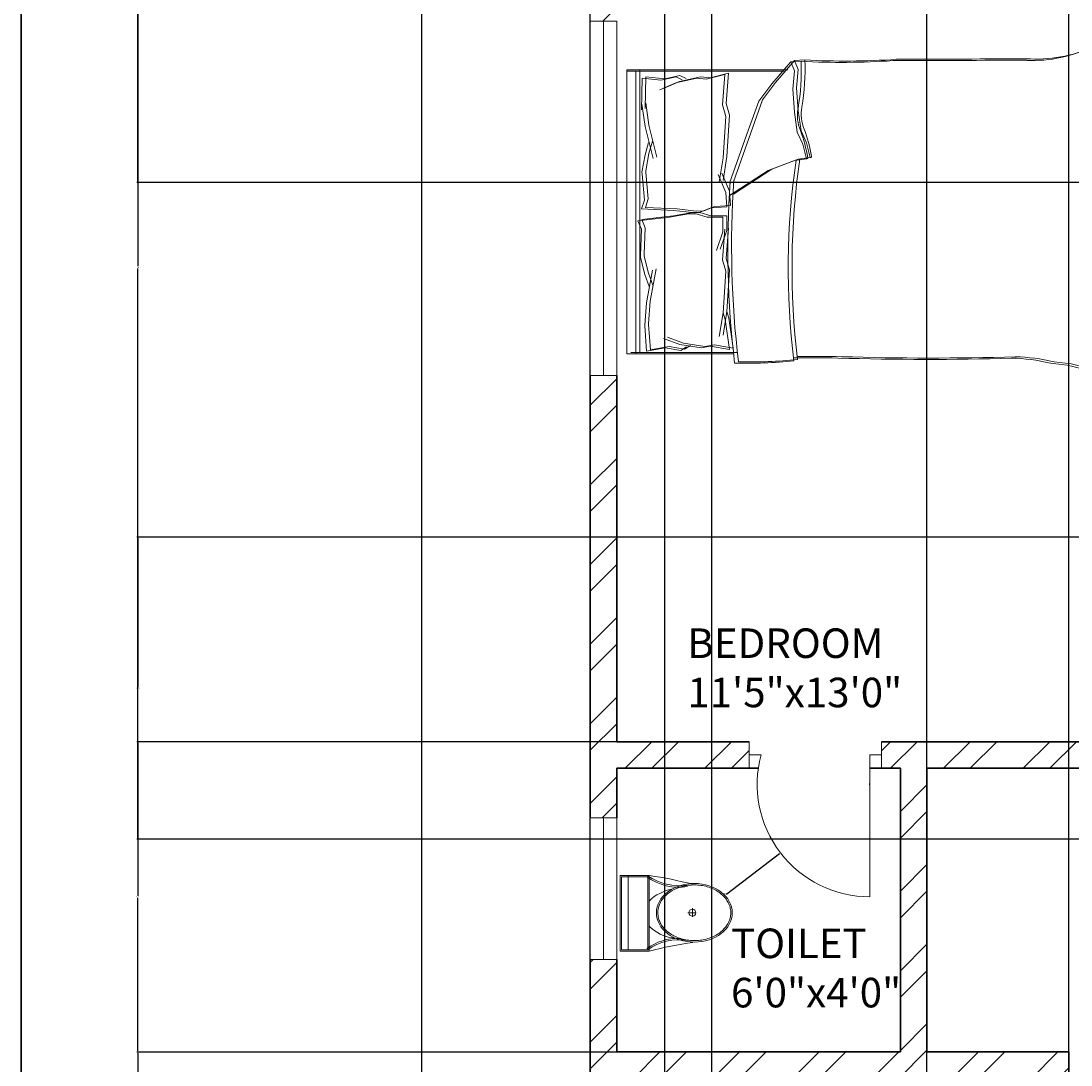
# Model space of a CAD drawing. Units: inches. Extents: x 2008 to 2657, y 1077 to 2165.
# Tile 10 of 16: x 2008 to 2186, y 1845 to 2022. Entities that reach past the tile are written whole.
import ezdxf

# ---------------------------------------------------------------- set-up
doc = ezdxf.new("R2010")
doc.units = ezdxf.units.IN
for name, color, linetype, lineweight in [('A-ANNO-DIMS', 2, 'Continuous', 18), ('A-ANNO-TTLB', 7, 'Continuous', 35), ('A-AREA-IDEN', 4, 'Continuous', 18), ('A-DOOR', 11, 'Continuous', 18), ('A-FLOR-FIXT', 8, 'Continuous', 18), ('A-FURN', 8, 'Continuous', 13), ('A-GLAZ', 191, 'Continuous', 18), ('A-WALL', 7, 'Continuous', 35)]:
    doc.layers.add(name, color=color, linetype=linetype, lineweight=lineweight)
doc.layers.add('A-WALL-PATT', color=30, linetype='Continuous', lineweight=13, true_color=0xf8991e)
doc.styles.get("Standard").update_dxf_attribs({"font": 'arial.ttf'})
doc.dimstyles.get("Standard").update_dxf_attribs({"dimtxt": 0.18, "dimasz": 0.18, "dimexe": 0.18, "dimexo": 0.0625, "dimgap": 0.09, "dimtad": 0, "dimtih": 1, "dimtoh": 1, "dimdec": 4, "dimzin": 0, "dimdsep": 46, "dimtxsty": 'Standard', "dimcen": 0.09, "dimadec": 0, "dimazin": 0, "dimtfac": 1, "dimtdec": 4, "dimtofl": 0, "dimtmove": 0, "dimatfit": 3, "dimfxl": 1, "dimtolj": 1, "dimtzin": 0, "dimarcsym": 0})

# ---------------------------------------------------------------- blocks, each defined once
blk = doc.blocks.new('A$C31115884')
for p, q in [((257.5, 466.4), (257.5, 523.2)), ((283.1, 497.7), (223.4, 497.7)), ((0, 200), (0, 0)), ((520, 200), (0, 200)), ((10, 190), (10, 10)), ((510, 190), (10, 190)), ((510, 10), (510, 190)), ((520, 0), (520, 200)), ((510, 54.5), (0, 54.5)), ((10, 10), (510, 10)), ((0, 0), (520, 0))]:
    blk.add_line(p, q)
blk.add_circle((255.6, 496.4), 23.6)
for centre, radius, start, end in [((2777.7, -204.6), 2807, 165.4549, 171.71327), ((-294.5, 403.3), 364.7, 324.20913, 9.34987), ((-294.5, 403.3), 374.7, 324.20913, 9.34987), ((805.8, 403.3), 364.7, 170.65013, 215.79087), ((3237, 905), 2807, 188.28673, 194.5451), ((139.5, 406.2), 293.5, 315.84364, 2.65635), ((805.8, 403.3), 374.7, 179.20365, 215.79087), ((383.6, 406.2), 293.5, 190.27735, 224.15636)]:
    blk.add_arc(centre, radius, start, end)
blk.add_ellipse((256.2, 509.9), major_axis=(0, -260.7), ratio=0.772727)
blk.add_open_spline([(256.2, 259.2), (263.1, 259.2), (270, 259.7), (287.8, 262.3), (298.7, 265.1), (319.9, 273.1), (330.2, 278.4), (350.1, 291.1), (359.7, 298.7), (377.7, 315.9), (386.2, 325.5), (401.7, 346.6), (408.8, 358.1), (421.3, 382.5), (426.8, 395.5), (435.9, 422.4), (439.5, 436.4), (444.8, 465.1), (446.5, 479.7), (447.9, 509.2), (447.6, 524), (445, 553.3), (442.7, 567.8), (436.3, 596), (432.1, 609.7), (421.9, 636), (416, 648.6), (402.5, 672.1), (395, 683), (378.6, 703), (369.8, 712.1), (351.1, 728), (341.3, 734.8), (320.9, 746.2), (310.4, 750.7), (288.9, 757.3), (278, 759.4), (256, 761), (245, 760.6), (223.1, 757.2), (212.3, 754.3), (191.1, 746.1), (180.8, 740.7), (160.9, 727.8), (151.4, 720.1), (133.5, 702.7), (125.1, 693), (109.6, 671.7), (102.6, 660.2), (90.2, 635.7), (84.9, 622.7), (76, 595.6), (72.4, 581.6), (67.2, 552.9), (65.6, 538.2), (64.4, 508.8), (64.8, 494), (67.5, 464.7), (69.9, 450.2), (76.6, 422), (80.8, 408.3), (91.1, 382.2), (97.2, 369.7), (110.8, 346.3), (118.4, 335.4), (134.8, 315.6), (143.7, 306.7), (162.4, 290.9), (172.3, 284.2), (192.8, 273), (203.3, 268.6), (224.8, 262.2), (235.8, 260.2), (249.9, 259.3), (253, 259.2), (256.2, 259.2)], degree=3, knots=[0, 0, 0, 0, 0.110105, 0.110105, 0.285049, 0.285049, 0.459994, 0.459994, 0.634938, 0.634938, 0.809882, 0.809882, 0.984827, 0.984827, 1.159771, 1.159771, 1.334715, 1.334715, 1.50966, 1.50966, 1.684604, 1.684604, 1.859549, 1.859549, 2.034493, 2.034493, 2.209437, 2.209437, 2.384382, 2.384382, 2.559326, 2.559326, 2.73427, 2.73427, 2.909215, 2.909215, 3.084159, 3.084159, 3.259103, 3.259103, 3.434048, 3.434048, 3.608992, 3.608992, 3.783936, 3.783936, 3.958881, 3.958881, 4.133825, 4.133825, 4.30877, 4.30877, 4.483714, 4.483714, 4.658658, 4.658658, 4.833603, 4.833603, 5.008547, 5.008547, 5.183491, 5.183491, 5.358436, 5.358436, 5.53338, 5.53338, 5.708324, 5.708324, 5.883269, 5.883269, 6.058213, 6.058213, 6.233158, 6.233158, 6.283185, 6.283185, 6.283185, 6.283185])
blk = doc.blocks.new('BED-DOUBLE')
for p, q in [((27.75, 52.87), (24.5, 49.16)), ((27.75, 52.87), (24.5, 49.16)), ((28.39, 53.1), (25.14, 49.39)), ((28.39, 53.1), (25.14, 49.39)), ((29.49, 52.95), (27.75, 52.87, 3.87)), ((29.49, 52.95), (27.75, 52.87, 3.87)), ((28.37, 51.33), (27.75, 52.87)), ((28.37, 51.33), (27.75, 52.87)), ((30.13, 53.18), (28.39, 53.1, 3.87)), ((30.13, 53.18), (28.39, 53.1, 3.87)), ((29, 51.56), (28.39, 53.1)), ((29, 51.56), (28.39, 53.1)), ((28.7, 48.46), (29, 51.56)), ((28.7, 48.46), (29, 51.56)), ((0, 51.49), (0.64, 51.49)), ((0, 3.48), (0, 51.49)), ((0, 51.27), (26.61, 51.27)), ((0, 51.27), (26.61, 51.27)), ((0.64, 51.49), (27.25, 51.49)), ((0.64, 51.49), (27.25, 51.49)), ((1.53, 3.48), (1.53, 51.27)), ((1.53, 3.48), (1.53, 51.27)), ((2.17, 3.7), (2.17, 51.49)), ((2.17, 3.7), (2.17, 51.49)), ((2.56, 50.11), (2.46, 44.71)), ((2.56, 50.11), (2.46, 44.71)), ((2.56, 50.11), (5.77, 49.73)), ((2.56, 50.11), (5.77, 49.73)), ((3.2, 50.34), (3.1, 44.94)), ((3.2, 50.34), (3.1, 44.94)), ((3.2, 50.34), (6.41, 49.96)), ((3.2, 50.34), (6.41, 49.96)), ((5.77, 49.73), (8.34, 50.33)), ((5.77, 49.73), (8.34, 50.33)), ((6.41, 49.96), (8.98, 50.56)), ((6.41, 49.96), (8.98, 50.56)), ((11.83, 50.11), (8.26, 49.31)), ((11.83, 50.11), (8.26, 49.31)), ((8.34, 50.33), (9.38, 49.82)), ((8.34, 50.33), (9.38, 49.81)), ((12.47, 50.34), (8.9, 49.54)), ((12.47, 50.34), (8.9, 49.54)), ((8.98, 50.56), (10.02, 50.04)), ((8.98, 50.56), (10.02, 50.04)), ((13.43, 49.92), (11.83, 50.11)), ((13.43, 49.92), (11.83, 50.11)), ((14.07, 50.15), (12.47, 50.34)), ((14.07, 50.15), (12.47, 50.34)), ((16.57, 50.7), (13.43, 49.92)), ((16.57, 50.7), (13.43, 49.92)), ((17.21, 50.93), (14.07, 50.15)), ((17.21, 50.93), (14.07, 50.15)), ((16.17, 45.57), (16.57, 50.7)), ((16.17, 45.57), (16.57, 50.7)), ((16.81, 45.8), (17.21, 50.93)), ((16.81, 45.8), (17.21, 50.93)), ((28.06, 48.23), (28.37, 51.33)), ((28.06, 48.23), (28.37, 51.33)), ((8.26, 49.31), (5.58, 48.13)), ((8.26, 49.31), (5.58, 48.13)), ((8.9, 49.54), (6.22, 48.36)), ((8.9, 49.54), (6.22, 48.36)), ((24.5, 49.16), (22.33, 46.22)), ((24.5, 49.16), (22.33, 46.22)), ((25.14, 49.39), (22.97, 46.45)), ((25.14, 49.39), (22.97, 46.45)), ((28.37, 44.36), (28.06, 48.23)), ((28.37, 44.36), (28.06, 48.23)), ((29, 44.59), (28.7, 48.46)), ((29, 44.59), (28.7, 48.46)), ((22.33, 46.22), (20.32, 40.64)), ((22.33, 46.22), (20.32, 40.64)), ((22.97, 46.45), (20.96, 40.87)), ((22.97, 46.45), (20.96, 40.87)), ((2.46, 44.71), (2.54, 45.71)), ((2.46, 44.71), (2.54, 45.71)), ((2.54, 45.71), (3.07, 41.91)), ((2.54, 45.71), (3.07, 41.91)), ((3.1, 44.94), (3.18, 45.94)), ((3.1, 44.94), (3.18, 45.94)), ((3.18, 45.94), (3.71, 42.14)), ((3.18, 45.94), (3.71, 42.14)), ((16.73, 43.61), (16.17, 45.57)), ((16.73, 43.61), (16.17, 45.57)), ((17.37, 43.84), (16.81, 45.8)), ((17.37, 43.83), (16.81, 45.8)), ((29.47, 41.18), (29, 44.59)), ((29.47, 41.18), (29, 44.59)), ((16.3, 36.6), (16.73, 43.61)), ((16.3, 36.6), (16.73, 43.61)), ((16.93, 36.83), (17.37, 43.84)), ((16.93, 36.82), (17.37, 43.83)), ((28.83, 40.95), (28.37, 44.36)), ((28.83, 40.95), (28.37, 44.36)), ((3.07, 41.91), (4.42, 36.5)), ((3.07, 41.91), (4.42, 36.5)), ((3.71, 42.14), (5.06, 36.72)), ((3.71, 42.14), (5.06, 36.72)), ((20.96, 40.87), (18.02, 32.54)), ((20.96, 40.87), (18.02, 32.53)), ((29.76, 38.94), (28.83, 40.95)), ((29.76, 38.94), (28.83, 40.95)), ((30.4, 39.17), (29.47, 41.18)), ((30.4, 39.17), (29.47, 41.18)), ((3.67, 39.2), (3.08, 37.14)), ((3.67, 39.2), (3.08, 37.14)), ((4.31, 39.43), (3.72, 37.36)), ((4.31, 39.43), (3.72, 37.36)), ((20.32, 40.64), (17.38, 32.31)), ((20.32, 40.64), (17.38, 32.31)), ((31.02, 36.69), (30.4, 39.17)), ((31.02, 36.69), (30.4, 39.17)), ((79.25, 15.06), (79.25, 39.68)), ((79.25, 15.06), (79.25, 39.68)), ((79.88, 15.29), (79.88, 39.91)), ((79.88, 15.29), (79.88, 39.91)), ((3.72, 37.36), (3.18, 34.43)), ((3.72, 37.36), (3.18, 34.43)), ((30.38, 36.46), (29.76, 38.94)), ((30.38, 36.46), (29.76, 38.94)), ((3.08, 37.14), (2.54, 34.21)), ((3.08, 37.14), (2.54, 34.2)), ((15.63, 32.56), (16.3, 36.6)), ((15.63, 32.56), (16.3, 36.6)), ((16.27, 32.79), (16.93, 36.83)), ((16.27, 32.79), (16.93, 36.82)), ((23.88, 34.45), (28.37, 36.15)), ((23.88, 34.45), (28.37, 36.15)), ((24.52, 34.68), (29, 36.38)), ((24.52, 34.68), (29, 36.38)), ((28.37, 36.15), (30.38, 36.46)), ((28.37, 36.15), (30.38, 36.46)), ((29, 36.38), (31.02, 36.69)), ((29, 36.38), (31.02, 36.69)), ((2.54, 34.21), (2.56, 33.88)), ((2.54, 34.2), (2.56, 33.88)), ((2.56, 33.88), (2.98, 29.46)), ((2.56, 33.88), (2.98, 29.46)), ((3.18, 34.43), (3.2, 34.11)), ((3.18, 34.43), (3.2, 34.11)), ((3.2, 34.11), (3.62, 29.68)), ((3.2, 34.11), (3.62, 29.68)), ((16.74, 30.75), (15.45, 33.82)), ((16.74, 30.75), (15.45, 33.82)), ((17.38, 30.98), (16.09, 34.05)), ((17.38, 30.98), (16.09, 34.05)), ((17.38, 30.26), (23.88, 34.45)), ((17.38, 30.26), (23.88, 34.45)), ((18.02, 30.49), (24.52, 34.68)), ((18.02, 30.49), (24.52, 34.68)), ((16.89, 28.3), (16.74, 30.75)), ((16.89, 28.3), (16.74, 30.75)), ((17.53, 28.53), (17.38, 30.98)), ((17.53, 28.53), (17.38, 30.98)), ((2.98, 29.46), (2.49, 27.98)), ((2.98, 29.46), (2.49, 27.98)), ((3.62, 29.68), (3.13, 28.21)), ((3.62, 29.68), (3.13, 28.21)), ((14.86, 28.36), (17.53, 28.53)), ((14.86, 28.36), (17.53, 28.53)), ((2.49, 27.98), (7.87, 27.73)), ((2.49, 27.98), (7.87, 27.73)), ((2.51, 26.21), (7.86, 26.79)), ((2.51, 26.21), (7.86, 26.79)), ((3.13, 28.21), (8.51, 27.96)), ((3.13, 28.21), (8.51, 27.96)), ((7.22, 26.56), (10.4, 27.14)), ((7.22, 26.56), (10.4, 27.14)), ((7.86, 26.79), (11.04, 27.37)), ((7.86, 26.79), (11.04, 27.37)), ((7.87, 27.73), (11.08, 27.36)), ((7.87, 27.73), (11.08, 27.36)), ((8.51, 27.96), (11.72, 27.58)), ((8.51, 27.96), (11.72, 27.58)), ((10.4, 27.14), (11.7, 27.14)), ((10.4, 27.14), (11.7, 27.14)), ((11.04, 27.37), (12.34, 27.37)), ((11.04, 27.37), (12.34, 27.37)), ((11.08, 27.36), (12.38, 27.44)), ((11.08, 27.36), (12.38, 27.44)), ((11.7, 27.14), (13.58, 26.56)), ((11.7, 27.14), (13.58, 26.56)), ((11.72, 27.58), (13.02, 27.66)), ((11.72, 27.58), (13.02, 27.66)), ((12.34, 27.37), (14.22, 26.79)), ((12.34, 27.37), (14.22, 26.79)), ((12.38, 27.44), (14.22, 28.13)), ((12.38, 27.44), (14.22, 28.13)), ((13.02, 27.66), (14.86, 28.36)), ((13.02, 27.66), (14.86, 28.36)), ((14.22, 28.13), (16.89, 28.3)), ((14.22, 28.13), (16.89, 28.3)), ((14.22, 26.79), (16.9, 26.79)), ((14.22, 26.79), (16.9, 26.79)), ((16.9, 26.79), (16.9, 24.33)), ((16.9, 26.79), (16.9, 24.33)), ((1.87, 25.98), (7.22, 26.56)), ((1.87, 25.98), (7.22, 26.56)), ((2.45, 24.54), (1.87, 25.98)), ((2.45, 24.54), (1.87, 25.98)), ((3.09, 24.77), (2.51, 26.21)), ((3.09, 24.77), (2.51, 26.21)), ((13.58, 26.56), (16.26, 26.56)), ((13.58, 26.56), (16.26, 26.56)), ((16.26, 26.56), (16.26, 24.1)), ((16.26, 26.56), (16.26, 24.1)), ((2.3, 20.09), (2.45, 24.54)), ((2.3, 20.09), (2.45, 24.54)), ((2.94, 20.32), (3.09, 24.77)), ((2.94, 20.32), (3.09, 24.77)), ((16.26, 24.1), (15.17, 20.96)), ((16.26, 24.1), (15.17, 20.96)), ((16.9, 24.33), (15.81, 21.19)), ((16.9, 24.33), (15.81, 21.19)), ((16.17, 19.38), (16.57, 24.52)), ((16.17, 19.38), (16.57, 24.52)), ((16.81, 19.61), (17.21, 24.74)), ((16.81, 19.61), (17.21, 24.74)), ((2.3, 19.77), (2.3, 20.09)), ((2.3, 19.77), (2.3, 20.09)), ((3.03, 16.88), (2.3, 19.77)), ((3.03, 16.88), (2.3, 19.77)), ((2.94, 20), (2.94, 20.32)), ((2.94, 20), (2.94, 20.32)), ((3.67, 17.11), (2.94, 20)), ((3.67, 17.11), (2.94, 20)), ((17.37, 17.65), (16.81, 19.61)), ((17.37, 17.65), (16.81, 19.61)), ((3.96, 12.34), (4.97, 17.83)), ((3.96, 12.34), (4.97, 17.83)), ((16.73, 17.42), (16.17, 19.38)), ((16.73, 17.42), (16.17, 19.38)), ((3.75, 14.86), (3.03, 16.88)), ((3.75, 14.86), (3.03, 16.88)), ((3.32, 12.11), (4.33, 17.6)), ((3.32, 12.11), (4.33, 17.6)), ((4.39, 15.08), (3.67, 17.11)), ((4.39, 15.08), (3.67, 17.11)), ((16.3, 10.41), (16.73, 17.42)), ((16.3, 10.41), (16.73, 17.42)), ((16.93, 10.64), (17.37, 17.65)), ((16.93, 10.64), (17.37, 17.65)), ((3.03, 8.29), (3.32, 12.11)), ((3.03, 8.29), (3.32, 12.11)), ((3.67, 8.51), (3.96, 12.34)), ((3.67, 8.51), (3.96, 12.34)), ((15.63, 6.38), (16.3, 10.41)), ((15.63, 6.38), (16.3, 10.41)), ((16.27, 6.61), (16.93, 10.64)), ((16.27, 6.61), (16.93, 10.64)), ((16.3, 10.41), (16.62, 9.28)), ((16.3, 10.41), (16.62, 9.28)), ((16.62, 9.28), (17.34, 4.18)), ((16.62, 9.28), (17.34, 4.18)), ((16.93, 10.64), (17.26, 9.51)), ((16.93, 10.64), (17.26, 9.51)), ((17.26, 9.51), (17.98, 4.41)), ((17.26, 9.51), (17.98, 4.41)), ((3.01, 8.18), (3.03, 8.29)), ((3.01, 8.18), (3.03, 8.29)), ((3.34, 3.9), (3.01, 8.18)), ((3.34, 3.9), (3.01, 8.18)), ((3.65, 8.41), (3.67, 8.51)), ((3.65, 8.41), (3.67, 8.51)), ((3.98, 4.13), (3.65, 8.41)), ((3.98, 4.13), (3.65, 8.41)), ((8.96, 5.05), (6.21, 6.06)), ((8.96, 5.05), (6.21, 6.06)), ((9.59, 5.28), (6.85, 6.29)), ((9.59, 5.28), (6.85, 6.29)), ((18.75, 3.7), (0.64, 3.7)), ((18.75, 3.7), (0.64, 3.7)), ((3.32, 3.9), (6.5, 4.47)), ((3.32, 3.89), (6.5, 4.47)), ((3.96, 4.12), (7.14, 4.7)), ((3.96, 4.12), (7.14, 4.7)), ((6.5, 4.47), (9.1, 4.04)), ((6.5, 4.47), (9.1, 4.04)), ((7.14, 4.7), (9.74, 4.27)), ((7.14, 4.7), (9.74, 4.27)), ((12.57, 4.47), (8.96, 5.05)), ((12.57, 4.47), (8.96, 5.05)), ((9.1, 4.04), (10.11, 4.62)), ((9.1, 4.04), (10.11, 4.62)), ((13.21, 4.7), (9.59, 5.28)), ((13.21, 4.7), (9.59, 5.28)), ((9.74, 4.27), (10.75, 4.85)), ((9.74, 4.27), (10.75, 4.85)), ((14.16, 4.76), (12.57, 4.47)), ((14.16, 4.76), (12.57, 4.47)), ((14.8, 4.99), (13.21, 4.7)), ((14.8, 4.99), (13.21, 4.7)), ((17.34, 4.18), (14.16, 4.76)), ((17.34, 4.18), (14.16, 4.76)), ((17.98, 4.41), (14.8, 4.99)), ((17.98, 4.41), (14.8, 4.99)), ((18.11, 3.48), (0, 3.48)), ((18.11, 3.48), (0, 3.48))]:
    blk.add_line(p, q)
for centre, radius, start, end in [((68.67, 76.16), 23.07, 267.4714, 296.4681), ((68.67, 76.16), 23.07, 267.4714, 296.4681), ((69.31, 76.39), 23.07, 267.4714, 296.4681), ((69.31, 76.39), 23.07, 267.4714, 296.4681), ((78.87, 54.41), 1.1, 332.6588, 86.02), ((78.87, 54.41), 1.1, 332.6588, 86.02), ((79.51, 54.64), 1.1, 332.6588, 86.02), ((79.51, 54.64), 1.1, 332.6588, 86.02), ((68.46, -4508.51), 4561.86, 90.00217, 90.28689), ((68.46, -4508.51), 4561.86, 90.00217, 90.28689), ((212.28, 41.15), 133.04, 174.4998, 180.6351), ((212.28, 41.15), 133.04, 174.4998, 180.6351), ((212.92, 41.38), 133.04, 174.4998, 180.6351), ((212.92, 41.38), 133.04, 174.4998, 180.6351), ((-6.66, 51.33), 36.18, 349.8763, 2.5657), ((-6.66, 51.33), 36.18, 349.8763, 2.5657), ((36.32, 182.27), 129.5, 266.9791, 273.8365), ((36.32, 182.27), 129.5, 266.9791, 273.8365), ((-6.02, 51.56), 36.18, 349.8763, 2.5657), ((-6.02, 51.56), 36.18, 349.8763, 2.5657), ((36.95, 182.49), 129.5, 266.9791, 273.8365), ((36.95, 182.49), 129.5, 266.9791, 273.8365), ((67.82, -4508.74), 4561.86, 90.00217, 90.28689), ((67.82, -4508.74), 4561.86, 90.00217, 90.28689), ((35.07, 43.74), 6.22, 168.6608, 203.7384), ((35.07, 43.74), 6.22, 168.6608, 203.7384), ((35.71, 43.97), 6.22, 168.6608, 203.7384), ((35.71, 43.97), 6.22, 168.6608, 203.7384), ((1.48, 31.15), 29.65, 10.6617, 19.8806), ((1.48, 31.15), 29.65, 10.6617, 19.8806), ((2.12, 31.38), 29.65, 10.6617, 19.8806), ((2.12, 31.38), 29.65, 10.6617, 19.8806), ((156.32, 17.76), 129.02, 171.7845, 186.9006), ((156.32, 17.76), 129.02, 171.7845, 186.9006), ((156.96, 17.98), 129.02, 171.7845, 186.9006), ((156.96, 17.98), 129.02, 171.7845, 186.9006), ((30.44, 36.64), 0.185, 250.2464, 1.1377), ((30.44, 36.64), 0.185, 250.2464, 1.1377), ((31.08, 36.87), 0.185, 250.2464, 1.1377), ((31.08, 36.86), 0.185, 250.2464, 1.1377), ((182.05, 21.36), 164.97, 176.0865, 186.7821), ((182.05, 21.36), 164.97, 176.0865, 186.7821), ((182.69, 21.59), 164.97, 176.0865, 186.7821), ((182.69, 21.59), 164.97, 176.0865, 186.7821), ((-23.71, -17.22), 106.46, 13.3832, 17.7053), ((-23.71, -17.22), 106.46, 13.3832, 17.7053), ((-23.07, -16.99), 106.46, 13.3832, 17.7053), ((-23.07, -16.99), 106.46, 13.3832, 17.7053), ((200.84, 21.43), 121.76, 182.9958, 189.4091), ((200.84, 21.43), 121.76, 182.9958, 189.4091), ((201.48, 21.66), 121.76, 182.9958, 189.4091), ((201.48, 21.66), 121.76, 182.9958, 189.4091), ((20.1, 85.16), 83.31, 268.7218, 275.604), ((20.1, 85.16), 83.31, 268.7218, 275.604), ((20.74, 85.39), 83.31, 268.7218, 275.604), ((20.74, 85.39), 83.31, 268.7218, 275.604), ((31.17, -167.31), 170.11, 88.4762, 91.0082), ((31.17, -167.31), 170.11, 88.4762, 91.0082), ((31.81, -167.08), 170.11, 88.4762, 91.0082), ((31.81, -167.08), 170.11, 88.4762, 91.0082), ((50.61, 484.82), 482.31, 268.2277, 271.7185), ((50.61, 484.82), 482.31, 268.2277, 271.7185), ((51.25, 485.05), 482.31, 268.2277, 271.7185), ((51.25, 485.05), 482.31, 268.2277, 271.7185), ((64.52, -26.9), 29.63, 76.0648, 88.9113), ((64.52, -26.9), 29.63, 76.0648, 88.9113), ((65.15, -26.67), 29.63, 76.0648, 88.9113), ((65.15, -26.67), 29.63, 76.0648, 88.9113), ((70.28, -21.66), 23.56, 67.9751, 86.652), ((70.28, -21.66), 23.56, 67.9751, 86.652), ((70.92, -21.43), 23.56, 67.9751, 86.652), ((70.92, -21.43), 23.56, 67.9751, 86.652), ((79.72, 1.09), 1.09, 236.1736, 23.4781), ((79.72, 1.09), 1.09, 236.1736, 23.4781), ((80.36, 1.32), 1.09, 236.1736, 23.4781), ((80.36, 1.32), 1.09, 236.1736, 23.4781)]:
    blk.add_arc(centre, radius, start, end)
blk = doc.blocks.new('WIN-60IN-B')
for p, q in [((0, 4.5), (0, 0)), ((0, 4.5), (60, 4.5)), ((60, 2.25), (60, 4.5)), ((60, 4.5), (60, 0)), ((0, 0), (0, 2.25)), ((0, 2.25), (60, 2.25)), ((60, 0), (0, 0))]:
    blk.add_line(p, q)
blk = doc.blocks.new('WIN-24IN-B')
for p, q in [((0, 24), (4.5, 24)), ((0, 24), (0, 0)), ((4.5, 24), (2.25, 24)), ((2.25, 24), (2.25, 0)), ((4.5, 0), (4.5, 24)), ((2.25, 0), (0, 0)), ((0, 0), (4.5, 0))]:
    blk.add_line(p, q)
blk = doc.blocks.new('*D33')
at = {"layer": 'A-ANNO-DIMS', "color": 0, "lineweight": -2, "transparency": 16777216}
for p, q in [((2076.26, 1667.3), (2076.26, 2142.9)), ((2104.76, 1667.3), (2104.76, 2142.9)), ((2076.44, 2142.72), (2090.19, 2142.72)), ((2104.58, 2142.72), (2090.84, 2142.72))]:
    blk.add_line(p, q, dxfattribs=at)
at = {"layer": 'A-ANNO-DIMS', "color": 0, "transparency": 16777216}
for points in [[(2076.44, 2142.75), (2076.44, 2142.69), (2076.26, 2142.72)], [(2104.58, 2142.75), (2104.58, 2142.69), (2104.76, 2142.72)]]:
    blk.add_solid(points, dxfattribs=at)
at = {"layer": 'Defpoints', "color": 0, "transparency": 16777216}
for p in [(2104.76, 2142.72), (2076.26, 1667.24), (2104.76, 1667.24)]:
    blk.add_point(p, dxfattribs=at)
at = {"layer": 'A-ANNO-DIMS', "color": 0, "transparency": 16777216, "insert": (2090.51, 2142.72), "char_height": 0.18, "attachment_point": 5}
blk.add_mtext('\\A1;28.5', dxfattribs=at)
blk = doc.blocks.new('*D45')
at = {"layer": 'A-ANNO-DIMS', "color": 0, "lineweight": -2, "transparency": 16777216}
for p, q in [((2109.2, 1847.17), (2028.03, 1847.17)), ((2028.21, 1846.99), (2028.21, 1791.44)), ((2028.21, 1735.52), (2028.21, 1791.08)), ((2109.2, 1735.34), (2028.03, 1735.34))]:
    blk.add_line(p, q, dxfattribs=at)
at = {"layer": 'A-ANNO-DIMS', "color": 0, "transparency": 16777216}
for points in [[(2028.18, 1846.99), (2028.24, 1846.99), (2028.21, 1847.17)], [(2028.18, 1735.52), (2028.24, 1735.52), (2028.21, 1735.34)]]:
    blk.add_solid(points, dxfattribs=at)
at = {"layer": 'Defpoints', "color": 0, "transparency": 16777216}
for p in [(2028.21, 1847.17), (2109.26, 1847.17), (2109.26, 1735.34)]:
    blk.add_point(p, dxfattribs=at)
at = {"layer": 'A-ANNO-DIMS', "color": 0, "transparency": 16777216, "insert": (2028.21, 1791.26), "char_height": 0.18, "attachment_point": 5}
blk.add_mtext('\\A1;111.83', dxfattribs=at)
blk = doc.blocks.new('*D46')
at = {"layer": 'A-ANNO-DIMS', "color": 0, "lineweight": -2, "transparency": 16777216}
for p, q in [((2109.2, 1899.67), (2028.03, 1899.67)), ((2028.21, 1899.49), (2028.21, 1873.61)), ((2028.21, 1847.35), (2028.21, 1873.24)), ((2109.2, 1847.17), (2028.03, 1847.17))]:
    blk.add_line(p, q, dxfattribs=at)
at = {"layer": 'A-ANNO-DIMS', "color": 0, "transparency": 16777216}
for points in [[(2028.18, 1899.49), (2028.24, 1899.49), (2028.21, 1899.67)], [(2028.18, 1847.35), (2028.24, 1847.35), (2028.21, 1847.17)]]:
    blk.add_solid(points, dxfattribs=at)
at = {"layer": 'Defpoints', "color": 0, "transparency": 16777216}
for p in [(2028.21, 1899.67), (2109.26, 1899.67), (2109.26, 1847.17)]:
    blk.add_point(p, dxfattribs=at)
at = {"layer": 'A-ANNO-DIMS', "color": 0, "transparency": 16777216, "insert": (2028.21, 1873.42), "char_height": 0.18, "attachment_point": 5}
blk.add_mtext('\\A1;52.5', dxfattribs=at)
blk = doc.blocks.new('*D47')
at = {"layer": 'A-ANNO-DIMS', "color": 0, "lineweight": -2, "transparency": 16777216}
for p, q in [((2109.2, 2060.17), (2028.03, 2060.17)), ((2028.21, 2059.99), (2028.21, 1980.11)), ((2028.21, 1899.85), (2028.21, 1979.74)), ((2109.2, 1899.67), (2028.03, 1899.67))]:
    blk.add_line(p, q, dxfattribs=at)
at = {"layer": 'A-ANNO-DIMS', "color": 0, "transparency": 16777216}
for points in [[(2028.18, 2059.99), (2028.24, 2059.99), (2028.21, 2060.17)], [(2028.18, 1899.85), (2028.24, 1899.85), (2028.21, 1899.67)]]:
    blk.add_solid(points, dxfattribs=at)
at = {"layer": 'Defpoints', "color": 0, "transparency": 16777216}
for p in [(2028.21, 2060.17), (2109.26, 2060.17), (2109.26, 1899.67)]:
    blk.add_point(p, dxfattribs=at)
at = {"layer": 'A-ANNO-DIMS', "color": 0, "transparency": 16777216, "insert": (2028.21, 1979.92), "char_height": 0.18, "attachment_point": 5}
blk.add_mtext('\\A1;160.5', dxfattribs=at)
blk = doc.blocks.new('*D54')
at = {"layer": 'A-ANNO-DIMS', "color": 0, "lineweight": -2, "transparency": 16777216}
for p, q in [((2161.76, 1514.3), (2161.76, 2142.9)), ((2185.76, 1514.3), (2185.76, 2142.9)), ((2161.94, 2142.72), (2173.54, 2142.72)), ((2185.58, 2142.72), (2173.98, 2142.72))]:
    blk.add_line(p, q, dxfattribs=at)
at = {"layer": 'A-ANNO-DIMS', "color": 0, "transparency": 16777216}
for points in [[(2161.94, 2142.75), (2161.94, 2142.69), (2161.76, 2142.72)], [(2185.58, 2142.75), (2185.58, 2142.69), (2185.76, 2142.72)]]:
    blk.add_solid(points, dxfattribs=at)
at = {"layer": 'Defpoints', "color": 0, "transparency": 16777216}
for p in [(2185.76, 2142.72), (2161.76, 1514.24), (2185.76, 1514.24)]:
    blk.add_point(p, dxfattribs=at)
at = {"layer": 'A-ANNO-DIMS', "color": 0, "transparency": 16777216, "insert": (2173.76, 2142.72), "char_height": 0.18, "attachment_point": 5}
blk.add_mtext('\\A1;24', dxfattribs=at)
blk = doc.blocks.new('*D63')
at = {"layer": 'A-ANNO-DIMS', "color": 0, "lineweight": -2, "transparency": 16777216}
for p, q in [((2117.38, 1662.8), (2117.38, 2142.9)), ((2125.38, 1662.8), (2125.38, 2142.9)), ((2117.56, 2142.72), (2121.23, 2142.72)), ((2125.2, 2142.72), (2121.53, 2142.72))]:
    blk.add_line(p, q, dxfattribs=at)
at = {"layer": 'A-ANNO-DIMS', "color": 0, "transparency": 16777216}
for points in [[(2117.56, 2142.75), (2117.56, 2142.69), (2117.38, 2142.72)], [(2125.2, 2142.75), (2125.2, 2142.69), (2125.38, 2142.72)]]:
    blk.add_solid(points, dxfattribs=at)
at = {"layer": 'Defpoints', "color": 0, "transparency": 16777216}
for p in [(2125.38, 2142.72), (2117.38, 1662.74), (2125.38, 1662.74)]:
    blk.add_point(p, dxfattribs=at)
at = {"layer": 'A-ANNO-DIMS', "color": 0, "transparency": 16777216, "insert": (2121.38, 2142.72), "char_height": 0.18, "attachment_point": 5}
blk.add_mtext('\\A1;8', dxfattribs=at)
blk = doc.blocks.new('*D66')
at = {"layer": 'A-ANNO-DIMS', "color": 0, "lineweight": -2, "transparency": 16777216}
for p, q in [((2572.2, 2055.67), (2028.03, 2055.67)), ((2028.21, 2055.49), (2028.21, 2025.16)), ((2028.21, 1994.47), (2028.21, 2024.8)), ((2572.2, 1994.29), (2028.03, 1994.29))]:
    blk.add_line(p, q, dxfattribs=at)
at = {"layer": 'A-ANNO-DIMS', "color": 0, "transparency": 16777216}
for points in [[(2028.18, 2055.49), (2028.24, 2055.49), (2028.21, 2055.67)], [(2028.18, 1994.47), (2028.24, 1994.47), (2028.21, 1994.29)]]:
    blk.add_solid(points, dxfattribs=at)
at = {"layer": 'Defpoints', "color": 0, "transparency": 16777216}
for p in [(2572.26, 2055.67), (2028.21, 1994.29), (2572.26, 1994.29)]:
    blk.add_point(p, dxfattribs=at)
at = {"layer": 'A-ANNO-DIMS', "color": 0, "transparency": 16777216, "insert": (2028.21, 2024.98), "char_height": 0.18, "attachment_point": 5}
blk.add_mtext('\\A1;61.39', dxfattribs=at)
blk = doc.blocks.new('*D67')
at = {"layer": 'A-ANNO-DIMS', "color": 0, "lineweight": -2, "transparency": 16777216}
for p, q in [((2572.2, 1934.29), (2028.03, 1934.29)), ((2028.21, 1934.11), (2028.21, 1908.91)), ((2028.21, 1883.35), (2028.21, 1908.55)), ((2572.2, 1883.17), (2028.03, 1883.17))]:
    blk.add_line(p, q, dxfattribs=at)
at = {"layer": 'A-ANNO-DIMS', "color": 0, "transparency": 16777216}
for points in [[(2028.18, 1934.11), (2028.24, 1934.11), (2028.21, 1934.29)], [(2028.18, 1883.35), (2028.24, 1883.35), (2028.21, 1883.17)]]:
    blk.add_solid(points, dxfattribs=at)
at = {"layer": 'Defpoints', "color": 0, "transparency": 16777216}
for p in [(2028.21, 1934.29), (2572.26, 1934.29), (2572.26, 1883.17)]:
    blk.add_point(p, dxfattribs=at)
at = {"layer": 'A-ANNO-DIMS', "color": 0, "transparency": 16777216, "insert": (2028.21, 1908.73), "char_height": 0.18, "attachment_point": 5}
blk.add_mtext('\\A1;51.11', dxfattribs=at)
blk = doc.blocks.new('*D82')
at = {"layer": 'A-ANNO-DIMS', "color": 0, "lineweight": -2, "transparency": 16777216}
for p, q in [((2152, 1892.49), (2152.18, 1892.49)), ((2152.09, 1892.4), (2152.09, 1892.58)), ((2127.89, 1873.92), (2136.82, 1880.77)), ((2127.71, 1873.92), (2127.89, 1873.92))]:
    blk.add_line(p, q, dxfattribs=at)
at = {"layer": 'A-ANNO-DIMS', "color": 0, "transparency": 16777216}
blk.add_solid([(2136.81, 1880.8), (2136.84, 1880.75), (2136.97, 1880.88)], dxfattribs=at)
at = {"layer": 'Defpoints', "color": 0, "transparency": 16777216}
for p in [(2152.09, 1892.49), (2136.97, 1880.88)]:
    blk.add_point(p, dxfattribs=at)
at = {"layer": 'A-ANNO-DIMS', "color": 0, "transparency": 16777216, "insert": (2127.23, 1873.92), "char_height": 0.18, "attachment_point": 5}
blk.add_mtext('\\A1;R19.06', dxfattribs=at)

msp = doc.modelspace()

# ---------------------------------------------------------------- hatches: boundary and pattern name
at = {"layer": 'A-WALL-PATT'}
h = msp.add_hatch(dxfattribs=at)
h.set_pattern_fill('ANSI32', color=256)
h.paths.add_polyline_path([(2109.2619, 2094.6743), (2104.7619, 2094.6743), (2104.7619, 2072.1743), (2104.7619, 2021.6151), (2109.2619, 2021.6151), (2109.2619, 2055.6743), (2126.1387, 2055.6743), (2126.1387, 2057.9243), (2126.1387, 2060.1743), (2109.2619, 2060.1743)])
h.paths.add_polyline_path([(2223.2494, 2057.9243), (2223.2494, 2060.1743), (2186.1387, 2060.1743), (2186.1387, 2055.6743), (2223.2494, 2055.6743)])
h.paths.add_polyline_path([(2250.7619, 2072.1743), (2250.7619, 2090.1743), (2250.7619, 2094.6743), (2246.2619, 2094.6743), (2246.2619, 2060.1743), (2242.7242, 2060.1743), (2242.7242, 2055.6743), (2246.2619, 2055.6743), (2246.2619, 1899.6743), (2242.7458, 1899.6743), (2242.7458, 1897.4243), (2242.7458, 1895.1743), (2246.2619, 1895.1743), (2246.2619, 1878.8745), (2248.5119, 1878.8745), (2250.7619, 1878.8745), (2250.7619, 1991.1743), (2250.7619, 2025.6743), (2257.6798, 2025.6743), (2257.6798, 2027.9243), (2257.6798, 2030.1743), (2250.7619, 2030.1743)])
h.paths.add_polyline_path([(2411.2619, 2031.6743), (2409.0119, 2031.6743), (2406.7619, 2031.6743), (2406.7619, 2030.1743), (2322.7619, 2030.1743), (2322.7619, 2053.3443), (2318.2619, 2053.3443), (2318.2619, 2030.1743), (2305.6798, 2030.1743), (2305.6798, 2025.6743), (2318.2619, 2025.6743), (2322.7619, 2025.6743), (2406.7619, 2025.6743), (2406.7619, 1995.6743), (2406.7619, 1847.2677), (2250.7619, 1847.2677), (2250.7619, 1850.9902), (2248.5119, 1850.9902), (2246.2619, 1850.9902), (2246.2619, 1847.1743), (2246.2619, 1842.7677), (2303.0015, 1842.7677), (2303.0015, 1667.2413), (2298.4208, 1667.2413), (2298.4208, 1662.7413), (2303.0015, 1662.7413), (2303.0015, 1649.8758), (2307.5015, 1649.8758), (2307.5015, 1842.7677), (2406.7619, 1842.7677), (2411.2619, 1842.7677), (2411.2619, 1878.6743), (2415.8196, 1878.6743), (2415.8196, 1880.9243), (2415.8196, 1883.1743), (2411.2619, 1883.1743)])
h.paths.add_polyline_path([(2411.2619, 2094.6743), (2406.7619, 2094.6743), (2318.2619, 2094.6743), (2318.2619, 2077.3443), (2322.7619, 2077.3443), (2322.7619, 2090.1743), (2406.7619, 2090.1743), (2406.7619, 2072.1743), (2406.7619, 2067.6743), (2406.7619, 2052.7524), (2411.2619, 2052.7524), (2411.2619, 2055.6743), (2414.9888, 2055.6743), (2414.9888, 2057.9243), (2414.9888, 2060.1743), (2411.2619, 2060.1743), (2411.2619, 2072.1743)])
h.paths.add_polyline_path([(2576.7619, 2072.1743), (2576.7619, 2094.6743), (2572.2619, 2094.6743), (2572.2619, 2060.1743), (2525.8113, 2060.1743), (2525.8113, 2055.6743), (2572.2619, 2055.6743), (2572.2619, 1994.289), (2576.7619, 1994.289)])
h.paths.add_polyline_path([(2465.8113, 2060.1743), (2436.2802, 2060.1743), (2436.2802, 2055.6743), (2465.8113, 2055.6743), (2465.8113, 2057.9243)])
h.paths.add_polyline_path([(2576.7619, 1934.289), (2574.5119, 1934.289), (2572.2619, 1934.289), (2572.2619, 1883.1743), (2447.7027, 1883.1743), (2447.7027, 1878.6743), (2459.7619, 1878.6743), (2459.7619, 1830.4982), (2464.2619, 1830.4982), (2464.2619, 1878.6743), (2572.2619, 1878.6743), (2572.2619, 1868.4883), (2576.7619, 1868.4883)])
h.paths.add_polyline_path([(2576.7619, 1832.4883), (2572.2619, 1832.4883), (2572.2619, 1806.6743), (2464.2619, 1806.6743), (2464.2619, 1809.6629), (2459.7619, 1809.6629), (2459.7619, 1802.1743), (2483.7619, 1802.1743), (2483.7619, 1778.1743), (2488.2619, 1778.1743), (2488.2619, 1802.1743), (2572.2619, 1802.1743), (2572.2619, 1793.6101), (2576.7619, 1793.6101)])
h.paths.add_polyline_path([(2576.7619, 1769.6101), (2572.2619, 1769.6101), (2572.2619, 1754.1743), (2488.2619, 1754.1743), (2488.2619, 1757.2675), (2486.0119, 1757.2675), (2483.7619, 1757.2675), (2483.7619, 1754.1743), (2447.4528, 1754.1743), (2447.4528, 1749.6743), (2483.7619, 1749.6743), (2572.2619, 1749.6743), (2572.2619, 1715.1837), (2576.7619, 1715.1837)])
h.paths.add_polyline_path([(2576.7619, 1655.1837), (2572.2619, 1655.1837), (2572.2619, 1617.6743), (2411.2619, 1617.6743), (2411.2619, 1749.6743), (2414.2827, 1749.6743), (2414.2827, 1754.1743), (2406.7619, 1754.1743), (2406.7619, 1749.6743), (2406.7619, 1617.6743), (2307.5015, 1617.6743), (2307.5015, 1621.0007), (2305.2515, 1621.0007), (2303.0015, 1621.0007), (2303.0015, 1609.6944), (2307.5015, 1609.6944), (2307.5015, 1613.1743), (2406.7619, 1613.1743), (2406.7619, 1476.6743), (2415.532, 1476.6743), (2415.532, 1478.9243), (2415.532, 1481.1743), (2411.2619, 1481.1743), (2411.2619, 1613.1743), (2572.2619, 1613.1743), (2572.2619, 1584.6086), (2576.7619, 1584.6086)])
h.paths.add_polyline_path([(2576.7619, 1524.6086), (2572.2619, 1524.6086), (2572.2619, 1481.1743), (2483.7619, 1481.1743), (2447.5119, 1481.1743), (2447.5119, 1476.6743), (2483.7619, 1476.6743), (2483.7619, 1473.5051), (2488.2619, 1473.5051), (2488.2619, 1476.6743), (2572.2619, 1476.6743), (2572.2619, 1469.5488), (2576.7619, 1469.5488)])
h.paths.add_polyline_path([(2576.7619, 1445.5488), (2572.2619, 1445.5488), (2572.2619, 1428.6743), (2488.2619, 1428.6743), (2488.2619, 1455.6743), (2486.0119, 1455.6743), (2483.7619, 1455.6743), (2483.7619, 1428.6743), (2459.7619, 1428.6743), (2459.7619, 1422.1519), (2464.2619, 1422.1519), (2464.2619, 1424.1743), (2572.2619, 1424.1743), (2572.2619, 1407.5685), (2576.7619, 1407.5685)])
h.paths.add_polyline_path([(2576.7619, 1371.5685), (2572.2619, 1371.5685), (2572.2619, 1352.1743), (2464.2619, 1352.1743), (2464.2619, 1403.1384), (2462.0119, 1403.1384), (2459.7619, 1403.1384), (2459.7619, 1352.1743), (2446.3194, 1352.1743), (2446.3194, 1347.6743), (2572.2619, 1347.6743), (2572.2619, 1321.0291), (2576.7619, 1321.0291)])
h.paths.add_polyline_path([(2462.703, 1227.6743), (2436.0298, 1227.6743), (2436.0298, 1225.4243), (2436.0298, 1223.1743), (2462.703, 1223.1743), (2462.703, 1225.4243)])
h.paths.add_polyline_path([(2576.7619, 1261.0291), (2574.5119, 1261.0291), (2572.2619, 1261.0291), (2572.2619, 1227.6743), (2522.703, 1227.6743), (2522.703, 1223.1743), (2572.2619, 1223.1743), (2572.2619, 1188.6743), (2576.7619, 1188.6743), (2576.7619, 1193.1743), (2576.7619, 1223.1743)])
h.paths.add_polyline_path([(2414.2823, 1227.6743), (2411.2619, 1227.6743), (2411.2619, 1267.1779), (2409.0119, 1267.1779), (2406.7619, 1267.1779), (2406.7619, 1227.6743), (2322.7619, 1227.6743), (2322.7619, 1244.3623), (2318.2619, 1244.3623), (2318.2619, 1223.1743), (2406.7619, 1223.1743), (2406.7619, 1193.1743), (2406.7619, 1188.6743), (2411.2619, 1188.6743), (2411.2619, 1193.1743), (2411.2619, 1223.1743), (2414.2823, 1223.1743)])
h.paths.add_polyline_path([(2411.2619, 1347.6743), (2414.702, 1347.6743), (2414.702, 1349.9243), (2414.702, 1352.1743), (2411.2619, 1352.1743), (2411.2619, 1416.7413), (2307.5015, 1416.7413), (2307.5015, 1579.8489), (2305.2515, 1579.8489), (2303.0015, 1579.8489), (2303.0015, 1566.7413), (2299.2719, 1566.7413), (2299.2719, 1562.2413), (2303.0015, 1562.2413), (2303.0015, 1416.7413), (2246.2619, 1416.7413), (2246.2619, 1409.8616), (2250.7619, 1409.8616), (2250.7619, 1412.2413), (2406.7619, 1412.2413), (2406.7619, 1292.1743), (2304.9703, 1292.1743), (2304.9703, 1287.6743), (2318.2619, 1287.6743), (2318.2619, 1268.3623), (2322.7619, 1268.3623), (2322.7619, 1287.6743), (2406.7619, 1287.6743), (2406.7619, 1285.4748), (2411.2619, 1285.4748)])
h.paths.add_polyline_path([(2109.2619, 1262.7482), (2104.7619, 1262.7482), (2104.7619, 1223.1743), (2104.7619, 1193.1743), (2104.7619, 1188.6743), (2109.2619, 1188.6743), (2109.2619, 1223.1743), (2126.7928, 1223.1743), (2126.7928, 1225.4243), (2126.7928, 1227.6743), (2109.2619, 1227.6743)])
h.paths.add_polyline_path([(2222.3268, 1227.6743), (2186.7928, 1227.6743), (2186.7928, 1223.1743), (2222.3268, 1223.1743)])
h.paths.add_polyline_path([(2250.7619, 1287.6743), (2256.9703, 1287.6743), (2256.9703, 1289.9243), (2256.9703, 1292.1743), (2250.7619, 1292.1743), (2250.7619, 1382.2078), (2248.5119, 1382.2078), (2246.2619, 1382.2078), (2246.2619, 1347.6743), (2246.2619, 1227.6743), (2242.6068, 1227.6743), (2242.6068, 1223.1743), (2246.2619, 1223.1743), (2246.2619, 1188.6743), (2250.7619, 1188.6743), (2250.7619, 1193.1743), (2250.7619, 1227.6743)])
h.paths.add_polyline_path([(2133.2619, 1349.9243), (2133.2619, 1352.1743), (2109.2619, 1352.1743), (2109.2619, 1375.2826), (2104.7619, 1375.2826), (2104.7619, 1322.7482), (2109.2619, 1322.7482), (2109.2619, 1347.6743), (2133.2619, 1347.6743)])
h.paths.add_polyline_path([(2210.2105, 1352.1743), (2161.7619, 1352.1743), (2161.7619, 1412.2413), (2185.7619, 1412.2413), (2185.7619, 1420.1851), (2183.5119, 1420.1851), (2181.2619, 1420.1851), (2181.2619, 1416.7413), (2109.2619, 1416.7413), (2109.2619, 1452.4006), (2104.7619, 1452.4006), (2104.7619, 1399.2826), (2109.2619, 1399.2826), (2109.2619, 1412.2413), (2157.2619, 1412.2413), (2157.2619, 1352.1743), (2154.3383, 1352.1743), (2154.3383, 1347.6743), (2210.2105, 1347.6743)])
h.paths.add_polyline_path([(2185.7619, 1514.2413), (2161.7619, 1514.2413), (2161.7619, 1518.1307), (2159.5119, 1518.1307), (2157.2619, 1518.1307), (2157.2619, 1514.2413), (2109.2619, 1514.2413), (2109.2619, 1528.997), (2107.0119, 1528.997), (2104.7619, 1528.997), (2104.7619, 1488.4006), (2109.2619, 1488.4006), (2109.2619, 1509.7413), (2181.2619, 1509.7413), (2181.2619, 1441.2042), (2185.7619, 1441.2042)])
h.paths.add_polyline_path([(2270.4025, 1566.7413), (2109.2619, 1566.7413), (2080.7619, 1566.7413), (2080.7619, 1586.5643), (2076.2619, 1586.5643), (2076.2619, 1562.2413), (2080.7619, 1562.2413), (2104.7619, 1562.2413), (2104.7619, 1552.997), (2109.2619, 1552.997), (2109.2619, 1562.2413), (2157.2619, 1562.2413), (2157.2619, 1538.2413), (2161.7619, 1538.2413), (2161.7619, 1562.2413), (2205.2619, 1562.2413), (2270.4025, 1562.2413)])
h.paths.add_polyline_path([(2131.6813, 1897.4243), (2131.6813, 1899.6743), (2109.2619, 1899.6743), (2109.2619, 1961.6151), (2104.7619, 1961.6151), (2104.7619, 1886.8042), (2109.2619, 1886.8042), (2109.2619, 1895.1743), (2131.6813, 1895.1743)])
h.paths.add_polyline_path([(2185.7619, 1847.1743), (2161.7619, 1847.1743), (2161.7619, 1895.1743), (2185.7619, 1895.1743), (2211.543, 1895.1743), (2211.543, 1897.4243), (2211.543, 1899.6743), (2154.0916, 1899.6743), (2154.0916, 1897.4243), (2154.0916, 1895.1743), (2157.2619, 1895.1743), (2157.2619, 1847.1743), (2109.2619, 1847.1743), (2109.2619, 1862.8042), (2104.7619, 1862.8042), (2104.7619, 1821.243), (2109.2619, 1821.243), (2109.2619, 1842.6743), (2181.2619, 1842.6743), (2181.2619, 1840.6763), (2185.7619, 1840.6763)])
h.paths.add_polyline_path([(2109.2619, 1785.243), (2104.7619, 1785.243), (2104.7619, 1715.4691), (2109.2619, 1715.4691), (2109.2619, 1730.8423), (2157.2619, 1730.8423), (2157.2619, 1727.6404), (2161.7619, 1727.6404), (2161.7619, 1730.8423), (2185.7619, 1730.8423), (2185.7619, 1822.1438), (2183.5119, 1822.1438), (2181.2619, 1822.1438), (2181.2619, 1735.3423), (2109.2619, 1735.3423)])
h.paths.add_polyline_path([(2109.2619, 1691.4691), (2104.7619, 1691.4691), (2104.7619, 1667.2413), (2076.2619, 1667.2413), (2076.2619, 1646.5643), (2080.7619, 1646.5643), (2080.7619, 1662.7413), (2109.2619, 1662.7413), (2271.4941, 1662.7413), (2271.4941, 1664.9913), (2271.4941, 1667.2413), (2181.2619, 1667.2413), (2161.7619, 1667.2413), (2161.7619, 1708.3752), (2159.5119, 1708.3752), (2157.2619, 1708.3752), (2157.2619, 1667.2413), (2109.2619, 1667.2413)])
h.paths.add_polyline_path([(2233.1467, 1747.4973), (2270.0737, 1747.4973), (2270.0737, 1766.1547), (2233.1467, 1766.1547)], flags=9)

# ---------------------------------------------------------------- linework, layer by layer
at = {"layer": 'A-ANNO-TTLB'}
msp.add_lwpolyline([(2008.4537, 2164.5615), (2657.4477, 2164.5615), (2657.4477, 1076.8888), (2008.4537, 1076.8888)], close=True, dxfattribs=at)
at = {"layer": 'A-DOOR'}
for p, q in [((2131.6813, 1899.6743), (2131.6813, 1895.1743)), ((2154.0916, 1895.1743), (2154.0916, 1899.6743)), ((2154.0916, 1899.6743), (2154.0916, 1897.4243)), ((2131.6813, 1895.1743), (2131.6813, 1897.4243)), ((2131.6813, 1897.4243), (2133.6813, 1897.4243)), ((2154.0916, 1897.4243), (2152.0916, 1897.4243)), ((2152.0916, 1897.4243), (2152.0916, 1873.4243))]:
    msp.add_line(p, q, dxfattribs=at)
msp.add_arc((2152.0916, 1892.4856), 19.0613, 164.983488, 270, dxfattribs=at)
at = {"layer": 'A-WALL'}
for p, q in [((2104.7619, 1961.6151), (2104.7619, 1886.8042)), ((2109.2619, 1961.6151), (2109.2619, 1899.6743)), ((2109.2619, 1899.6743), (2131.6813, 1899.6743)), ((2109.2619, 1899.6743), (2131.6813, 1899.6743)), ((2154.0916, 1899.6743), (2156.5945, 1899.6743)), ((2154.0916, 1899.6743), (2213.0027, 1899.6743)), ((2109.2619, 1895.1743), (2133.2209, 1895.1743)), ((2109.2619, 1895.1743), (2109.2619, 1886.8042)), ((2109.2619, 1895.1743), (2133.2209, 1895.1743)), ((2152.0916, 1895.1743), (2157.2619, 1895.1743)), ((2152.0916, 1895.1743), (2157.2619, 1895.1743)), ((2157.2619, 1847.1743), (2157.2619, 1895.1743)), ((2161.7619, 1847.1743), (2161.7619, 1895.1743)), ((2161.7619, 1895.1743), (2185.7619, 1895.1743)), ((2185.7619, 1895.1743), (2211.543, 1895.1743)), ((2104.7619, 1862.8042), (2104.7619, 1821.243)), ((2109.2619, 1862.8042), (2109.2619, 1847.1743)), ((2109.2619, 1847.1743), (2157.2619, 1847.1743)), ((2161.7619, 1847.1743), (2185.7619, 1847.1743)), ((2185.7619, 1840.6763), (2185.7619, 1847.1743))]:
    msp.add_line(p, q, dxfattribs=at)

# ---------------------------------------------------------------- block references
at = {"layer": 'A-FLOR-FIXT', "xscale": 0.0246256636748975, "yscale": 0.0246256636748975, "zscale": 0.0246256636748975, "rotation": 270}
msp.add_blockref('A$C31115884', (2109.8376, 1877.0339), dxfattribs=at)
at = {"layer": 'A-FURN'}
msp.add_blockref('BED-DOUBLE', (2110.986, 1961.847), dxfattribs=at)
at = {"layer": 'A-GLAZ', "rotation": 89.99999999999832}
msp.add_blockref('WIN-60IN-B', (2109.2622, 1961.6153), dxfattribs=at)
at = {"layer": 'A-GLAZ'}
msp.add_blockref('WIN-24IN-B', (2104.762, 1862.804), dxfattribs=at)

# ---------------------------------------------------------------- texts
at = {"layer": 'A-AREA-IDEN', "char_height": 5, "attachment_point": 1}
for s, width, insert in [('BEDROOM\\P11\'5"x13\'0"', 112.074878, (2121.2071, 1918.8378)), ('TOILET\\P6\'0"x4\'0"', 131.844697, (2128.6069, 1868.0535))]:
    msp.add_mtext_dynamic_manual_height_columns(s, width=width, gutter_width=12.5, heights=[0], dxfattribs=dict(at, insert=insert))

# ---------------------------------------------------------------- dimensions: what is measured, and where the dimension line sits
at = {"layer": 'A-ANNO-DIMS'}
for base, p1, p2, override, picture, middle in [((2104.7619, 2142.7243), (2076.2619, 1667.2413), (2104.7619, 1667.2413), {"dimdec": 1, "dimlfac": 1, "dimrnd": 0, "dimzin": 0, "dimdsep": 46, "dimlunit": 2}, '*D33', (2090.5119, 2142.7243)), ((2125.3789, 2142.7243), (2117.3789, 1662.7413), (2125.3789, 1662.7413), {"dimdec": 0, "dimlfac": 1, "dimrnd": 0, "dimzin": 0, "dimdsep": 46, "dimlunit": 2}, '*D63', (2121.3789, 2142.7243)), ((2185.7619, 2142.7243), (2161.7619, 1514.2413), (2185.7619, 1514.2413), {"dimdec": 0, "dimlfac": 1, "dimrnd": 0, "dimzin": 0, "dimdsep": 46, "dimlunit": 2}, '*D54', (2173.7619, 2142.7243))]:
    dim = msp.add_linear_dim(base=base, p1=p1, p2=p2, dimstyle='Standard', override=override, dxfattribs=at)
    dim.commit()
    dim.dimension.update_dxf_attribs({"geometry": picture, "text_midpoint": middle})
for base, p1, p2, override, picture, middle in [((2028.2119, 2060.1743), (2109.2619, 1899.6743), (2109.2619, 2060.1743), {"dimdec": 1, "dimlfac": 1, "dimrnd": 0, "dimzin": 0, "dimdsep": 46, "dimlunit": 2}, '*D47', (2028.2119, 1979.9243)), ((2028.2119, 1994.289), (2572.2619, 2055.6743), (2572.2619, 1994.289), {"dimdec": 2, "dimlfac": 1, "dimrnd": 0, "dimzin": 0, "dimdsep": 46, "dimlunit": 2}, '*D66', (2028.2119, 2024.9817)), ((2028.2119, 1934.289), (2572.2619, 1883.1743), (2572.2619, 1934.289), {"dimdec": 2, "dimlfac": 1, "dimrnd": 0, "dimzin": 0, "dimdsep": 46, "dimlunit": 2}, '*D67', (2028.2119, 1908.7317)), ((2028.2119, 1899.6743), (2109.2619, 1847.1743), (2109.2619, 1899.6743), {"dimdec": 1, "dimlfac": 1, "dimrnd": 0, "dimzin": 0, "dimdsep": 46, "dimlunit": 2}, '*D46', (2028.2119, 1873.4243)), ((2028.2119, 1847.1743), (2109.2619, 1735.3423), (2109.2619, 1847.1743), {"dimdec": 2, "dimlfac": 1, "dimrnd": 0, "dimzin": 0, "dimdsep": 46, "dimlunit": 2}, '*D45', (2028.2119, 1791.2583))]:
    dim = msp.add_linear_dim(base=base, p1=p1, p2=p2, angle=90, dimstyle='Standard', override=override, dxfattribs=at)
    dim.commit()
    dim.dimension.update_dxf_attribs({"geometry": picture, "text_midpoint": middle})
dim = msp.add_radius_dim(center=(2152.0916, 1892.4856), mpoint=(2136.9678, 1880.8838), dimstyle='Standard', override={"dimdec": 2, "dimlfac": 1, "dimrnd": 0, "dimzin": 0, "dimdsep": 46, "dimlunit": 2}, dxfattribs=at)
dim.commit()
dim.dimension.update_dxf_attribs({"geometry": '*D82', "text_midpoint": (2127.2337, 1873.9228), "dimtype": 164})

doc.saveas('drawing.dxf')
